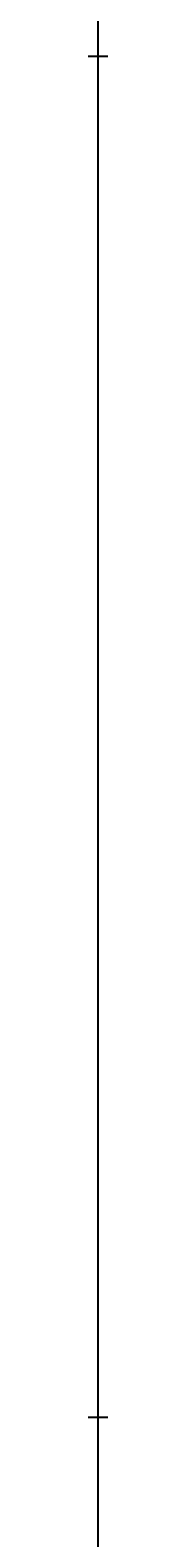
# Model space of a CAD drawing. Units: inches. Extents: x 35362 to 73946, y 43607 to 67532.
# Tile 31 of 134: x 48373 to 48373, y 46091 to 46564. Entities that reach past the tile are written whole.
import ezdxf

# ---------------------------------------------------------------- set-up
doc = ezdxf.new("R2010")
doc.units = ezdxf.units.IN
doc.header["$MEASUREMENT"] = 0
doc.layers.add('A-ANNO-DIMS', color=2, linetype='Continuous', lineweight=18)
doc.styles.get("Standard").update_dxf_attribs({"font": 'arial.ttf'})
doc.dimstyles.get("Standard").update_dxf_attribs({"dimtxt": 0.18, "dimasz": 0.18, "dimexe": 0.18, "dimexo": 0.0625, "dimgap": 0.09, "dimtad": 0, "dimtih": 1, "dimtoh": 1, "dimdec": 4, "dimzin": 0, "dimdsep": 46, "dimtxsty": 'Standard', "dimcen": 0.09, "dimadec": 0, "dimazin": 0, "dimtfac": 1, "dimtdec": 4, "dimtofl": 0, "dimtmove": 0, "dimatfit": 3, "dimfxl": 1, "dimtolj": 1, "dimtzin": 0, "dimarcsym": 0})

# ---------------------------------------------------------------- blocks, each defined once
blk = doc.blocks.new('*D5')
at = {"layer": 'A-ANNO-DIMS', "color": 0, "lineweight": -2, "transparency": 16777216}
for p, q in [((37121.95, 46919.32), (37121.95, 43606.68)), ((69871.5, 45449.83), (69871.5, 43606.68)), ((37122.13, 43606.86), (53496.29, 43606.86)), ((69871.32, 43606.86), (53497.15, 43606.86))]:
    blk.add_line(p, q, dxfattribs=at)
at = {"layer": 'A-ANNO-DIMS', "color": 0, "transparency": 16777216}
for points in [[(37122.13, 43606.89), (37122.13, 43606.83), (37121.95, 43606.86)], [(69871.32, 43606.89), (69871.32, 43606.83), (69871.5, 43606.86)]]:
    blk.add_solid(points, dxfattribs=at)
at = {"layer": 'Defpoints', "color": 0, "transparency": 16777216}
for p in [(37121.95, 46919.38), (69871.5, 45449.89), (69871.5, 43606.86)]:
    blk.add_point(p, dxfattribs=at)
at = {"layer": 'A-ANNO-DIMS', "color": 0, "transparency": 16777216, "insert": (53496.72, 43606.86), "char_height": 0.18, "attachment_point": 5}
blk.add_mtext('\\A1;32750', dxfattribs=at)
blk = doc.blocks.new('*D11')
at = {"layer": 'A-ANNO-DIMS', "color": 0, "lineweight": -2, "transparency": 16777216}
for p, q in [((47978.66, 56028.77), (47978.66, 43606.68)), ((53109.76, 56028.77), (53109.76, 43606.68)), ((47978.84, 43606.86), (50543.87, 43606.86)), ((53109.58, 43606.86), (50544.55, 43606.86))]:
    blk.add_line(p, q, dxfattribs=at)
at = {"layer": 'A-ANNO-DIMS', "color": 0, "transparency": 16777216}
for points in [[(47978.84, 43606.89), (47978.84, 43606.83), (47978.66, 43606.86)], [(53109.58, 43606.89), (53109.58, 43606.83), (53109.76, 43606.86)]]:
    blk.add_solid(points, dxfattribs=at)
at = {"layer": 'Defpoints', "color": 0, "transparency": 16777216}
for p in [(47978.66, 56028.84), (53109.76, 56028.84), (53109.76, 43606.86)]:
    blk.add_point(p, dxfattribs=at)
at = {"layer": 'A-ANNO-DIMS', "color": 0, "transparency": 16777216, "insert": (50544.21, 43606.86), "char_height": 0.18, "attachment_point": 5}
blk.add_mtext('\\A1;5131', dxfattribs=at)
blk = doc.blocks.new('*D27')
at = {"layer": 'A-ANNO-DIMS', "color": 0, "lineweight": -2, "transparency": 16777216}
for p, q in [((47978.66, 56028.77), (47978.66, 43606.68)), ((48373.49, 53428.96), (48373.49, 43606.68)), ((47978.84, 43606.86), (48175.68, 43606.86)), ((48373.31, 43606.86), (48176.47, 43606.86))]:
    blk.add_line(p, q, dxfattribs=at)
at = {"layer": 'A-ANNO-DIMS', "color": 0, "transparency": 16777216}
for points in [[(47978.84, 43606.89), (47978.84, 43606.83), (47978.66, 43606.86)], [(48373.31, 43606.89), (48373.31, 43606.83), (48373.49, 43606.86)]]:
    blk.add_solid(points, dxfattribs=at)
at = {"layer": 'Defpoints', "color": 0, "transparency": 16777216}
for p in [(47978.66, 56028.84), (48373.49, 53429.02), (48373.49, 43606.86)]:
    blk.add_point(p, dxfattribs=at)
at = {"layer": 'A-ANNO-DIMS', "color": 0, "transparency": 16777216, "insert": (48176.08, 43606.86), "char_height": 0.18, "attachment_point": 5}
blk.add_mtext('\\A1;394.8', dxfattribs=at)
blk = doc.blocks.new('*D67')
at = {"layer": 'A-ANNO-DIMS', "color": 0, "lineweight": -2, "transparency": 16777216}
for p, q in [((56873.54, 53351.53), (35361.77, 53351.53)), ((35361.95, 53351.35), (35361.95, 49400.89)), ((35361.95, 45450.07), (35361.95, 49400.53)), ((53793.58, 45449.89), (35361.77, 45449.89))]:
    blk.add_line(p, q, dxfattribs=at)
at = {"layer": 'A-ANNO-DIMS', "color": 0, "transparency": 16777216}
for points in [[(35361.92, 53351.35), (35361.98, 53351.35), (35361.95, 53351.53)], [(35361.92, 45450.07), (35361.98, 45450.07), (35361.95, 45449.89)]]:
    blk.add_solid(points, dxfattribs=at)
at = {"layer": 'Defpoints', "color": 0, "transparency": 16777216}
for p in [(35361.95, 53351.53), (56873.6, 53351.53), (53793.64, 45449.89)]:
    blk.add_point(p, dxfattribs=at)
at = {"layer": 'A-ANNO-DIMS', "color": 0, "transparency": 16777216, "insert": (35361.95, 49400.71), "char_height": 0.18, "attachment_point": 5}
blk.add_mtext('\\A1;7901.6', dxfattribs=at)
blk = doc.blocks.new('*D76')
at = {"layer": 'A-ANNO-DIMS', "color": 0, "lineweight": -2, "transparency": 16777216}
for p, q in [((54052.84, 46555.29), (35361.77, 46555.29)), ((35361.95, 46555.11), (35361.95, 46342.27)), ((35361.95, 46129.06), (35361.95, 46341.9)), ((53793.58, 46128.88), (35361.77, 46128.88))]:
    blk.add_line(p, q, dxfattribs=at)
at = {"layer": 'A-ANNO-DIMS', "color": 0, "transparency": 16777216}
for points in [[(35361.92, 46555.11), (35361.98, 46555.11), (35361.95, 46555.29)], [(35361.92, 46129.06), (35361.98, 46129.06), (35361.95, 46128.88)]]:
    blk.add_solid(points, dxfattribs=at)
at = {"layer": 'Defpoints', "color": 0, "transparency": 16777216}
for p in [(35361.95, 46555.29), (54052.9, 46555.29), (53793.64, 46128.88)]:
    blk.add_point(p, dxfattribs=at)
at = {"layer": 'A-ANNO-DIMS', "color": 0, "transparency": 16777216, "insert": (35361.95, 46342.09), "char_height": 0.18, "attachment_point": 5}
blk.add_mtext('\\A1;426.4', dxfattribs=at)
blk = doc.blocks.new('*D90')
at = {"layer": 'A-ANNO-DIMS', "color": 0, "lineweight": -2, "transparency": 16777216}
for p, q in [((53707.72, 47291.29), (35361.77, 47291.29)), ((35361.95, 47291.11), (35361.95, 46710.26)), ((35361.95, 46129.06), (35361.95, 46709.9)), ((53793.58, 46128.88), (35361.77, 46128.88))]:
    blk.add_line(p, q, dxfattribs=at)
at = {"layer": 'A-ANNO-DIMS', "color": 0, "transparency": 16777216}
for points in [[(35361.92, 47291.11), (35361.98, 47291.11), (35361.95, 47291.29)], [(35361.92, 46129.06), (35361.98, 46129.06), (35361.95, 46128.88)]]:
    blk.add_solid(points, dxfattribs=at)
at = {"layer": 'Defpoints', "color": 0, "transparency": 16777216}
for p in [(53707.78, 47291.29), (35361.95, 46128.88), (53793.64, 46128.88)]:
    blk.add_point(p, dxfattribs=at)
at = {"layer": 'A-ANNO-DIMS', "color": 0, "transparency": 16777216, "insert": (35361.95, 46710.08), "char_height": 0.18, "attachment_point": 5}
blk.add_mtext('\\A1;1162.4', dxfattribs=at)

msp = doc.modelspace()

# ---------------------------------------------------------------- dimensions: what is measured, and where the dimension line sits
at = {"layer": 'A-ANNO-DIMS'}
for base, p1, p2, override, picture, middle in [((53109.76, 43606.859), (47978.665, 56028.836), (53109.76, 56028.836), {"dimdec": 0, "dimlfac": 1, "dimrnd": 0, "dimzin": 0, "dimdsep": 46, "dimlunit": 2}, '*D11', (50544.212, 43606.859)), ((48373.492, 43606.859), (47978.665, 56028.836), (48373.492, 53429.019), {"dimdec": 1, "dimlfac": 1, "dimrnd": 0, "dimzin": 0, "dimdsep": 46, "dimlunit": 2}, '*D27', (48176.078, 43606.859)), ((69871.496, 43606.859), (37121.949, 46919.381), (69871.496, 45449.894), {"dimdec": 0, "dimlfac": 1, "dimrnd": 0, "dimzin": 0, "dimdsep": 46, "dimlunit": 2}, '*D5', (53496.723, 43606.859))]:
    dim = msp.add_linear_dim(base=base, p1=p1, p2=p2, dimstyle='Standard', override=override, dxfattribs=at)
    dim.commit()
    dim.dimension.update_dxf_attribs({"geometry": picture, "text_midpoint": middle})
for base, p1, p2, picture, middle in [((35361.949, 53351.529), (53793.638, 45449.894), (56873.602, 53351.529), '*D67', (35361.949, 49400.712)), ((35361.949, 46128.878), (53707.781, 47291.285), (53793.638, 46128.878), '*D90', (35361.949, 46710.081)), ((35361.949, 46555.293), (53793.638, 46128.878), (54052.899, 46555.293), '*D76', (35361.949, 46342.086))]:
    dim = msp.add_linear_dim(base=base, p1=p1, p2=p2, angle=90, dimstyle='Standard', override={"dimdec": 1, "dimlfac": 1, "dimrnd": 0, "dimzin": 0, "dimdsep": 46, "dimlunit": 2}, dxfattribs=at)
    dim.commit()
    dim.dimension.update_dxf_attribs({"geometry": picture, "text_midpoint": middle})

doc.saveas('drawing.dxf')
